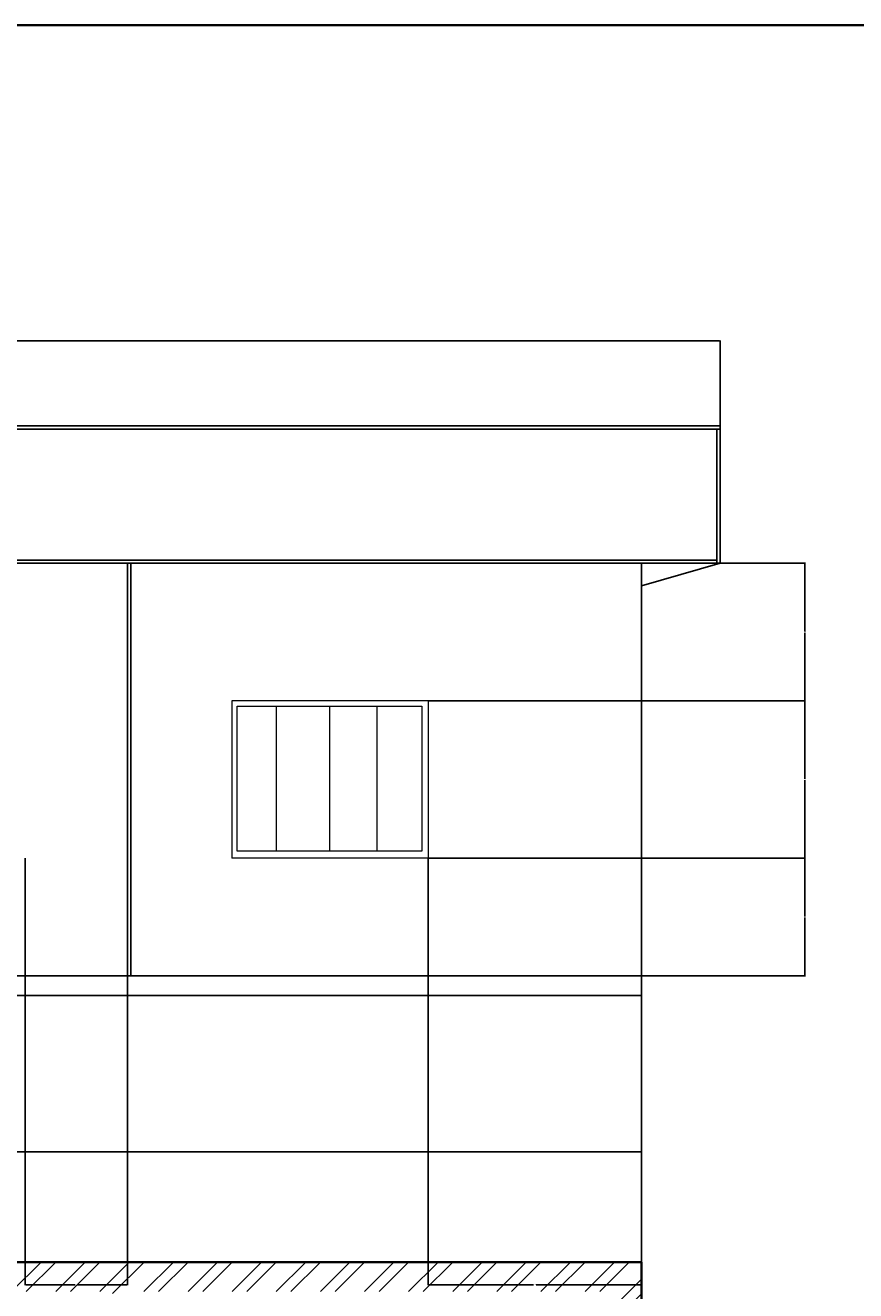
# Model space of a CAD drawing. Units: inches. Extents: x 1152 to 2588, y 1459 to 2618.
# Tile 14 of 17: x 1548 to 1802, y 2231 to 2618. Entities that reach past the tile are written whole.
import ezdxf

# ---------------------------------------------------------------- set-up
doc = ezdxf.new("R2010")
doc.units = ezdxf.units.IN
for name, color, linetype, lineweight in [('A-ANNO-DIMS', 2, 'Continuous', 18), ('A-ANNO-TTLB', 7, 'Continuous', 35), ('A-ELEV', 7, 'Continuous', 25), ('A-GLAZ', 4, 'Continuous', 18), ('A-WALL', 7, 'Continuous', 35), ('A-WALL-PATT', 8, 'Continuous', 13)]:
    doc.layers.add(name, color=color, linetype=linetype, lineweight=lineweight)
doc.styles.get("Standard").update_dxf_attribs({"font": 'arial.ttf'})
doc.dimstyles.get("Standard").update_dxf_attribs({"dimtxt": 0.18, "dimasz": 0.18, "dimexe": 0.18, "dimexo": 0.0625, "dimgap": 0.09, "dimtad": 0, "dimtih": 1, "dimtoh": 1, "dimdec": 4, "dimzin": 0, "dimdsep": 46, "dimtxsty": 'Standard', "dimcen": 0.09, "dimadec": 0, "dimazin": 0, "dimtfac": 1, "dimtdec": 4, "dimtofl": 0, "dimtmove": 0, "dimatfit": 3, "dimfxl": 1, "dimtolj": 1, "dimtzin": 0, "dimarcsym": 0})

# ---------------------------------------------------------------- blocks, each defined once
blk = doc.blocks.new('*D70')
at = {"layer": 'A-ANNO-DIMS', "color": 0, "lineweight": -2, "transparency": 16777216}
for p, q in [((1276.42, 2240.11), (1276.42, 2273.83)), ((1276.6, 2273.65), (1506.12, 2273.65)), ((1736.24, 2273.65), (1506.71, 2273.65)), ((1736.42, 2240.11), (1736.42, 2273.83))]:
    blk.add_line(p, q, dxfattribs=at)
at = {"layer": 'A-ANNO-DIMS', "color": 0, "transparency": 16777216}
for points in [[(1276.6, 2273.68), (1276.6, 2273.62), (1276.42, 2273.65)], [(1736.24, 2273.68), (1736.24, 2273.62), (1736.42, 2273.65)]]:
    blk.add_solid(points, dxfattribs=at)
at = {"layer": 'Defpoints', "color": 0, "transparency": 16777216}
for p in [(1736.42, 2273.65), (1276.42, 2240.05), (1736.42, 2240.05)]:
    blk.add_point(p, dxfattribs=at)
at = {"layer": 'A-ANNO-DIMS', "color": 0, "transparency": 16777216, "insert": (1506.42, 2273.65), "char_height": 0.18, "attachment_point": 5}
blk.add_mtext('\\A1;460', dxfattribs=at)
blk = doc.blocks.new('*D88')
at = {"layer": 'A-ANNO-DIMS', "color": 0, "lineweight": -2, "transparency": 16777216}
for p, q in [((1252.42, 2495.45), (1252.42, 2521.47)), ((1252.6, 2521.29), (1506.13, 2521.29)), ((1760.24, 2521.29), (1506.71, 2521.29)), ((1760.42, 2495.45), (1760.42, 2521.47))]:
    blk.add_line(p, q, dxfattribs=at)
at = {"layer": 'A-ANNO-DIMS', "color": 0, "transparency": 16777216}
for points in [[(1252.6, 2521.32), (1252.6, 2521.26), (1252.42, 2521.29)], [(1760.24, 2521.32), (1760.24, 2521.26), (1760.42, 2521.29)]]:
    blk.add_solid(points, dxfattribs=at)
at = {"layer": 'Defpoints', "color": 0, "transparency": 16777216}
for p in [(1760.42, 2521.29), (1252.42, 2495.39), (1760.42, 2495.39)]:
    blk.add_point(p, dxfattribs=at)
at = {"layer": 'A-ANNO-DIMS', "color": 0, "transparency": 16777216, "insert": (1506.42, 2521.29), "char_height": 0.18, "attachment_point": 5}
blk.add_mtext('\\A1;508', dxfattribs=at)
blk = doc.blocks.new('*D94')
at = {"layer": 'A-ANNO-DIMS', "color": 0, "lineweight": -2, "transparency": 16777216}
for p, q in [((1548.24, 2363.33), (1548.24, 2232.94)), ((1579.42, 2327.33), (1579.42, 2232.94)), ((1548.42, 2233.12), (1563.43, 2233.12)), ((1579.24, 2233.12), (1564.22, 2233.12))]:
    blk.add_line(p, q, dxfattribs=at)
at = {"layer": 'A-ANNO-DIMS', "color": 0, "transparency": 16777216}
for points in [[(1548.42, 2233.15), (1548.42, 2233.09), (1548.24, 2233.12)], [(1579.24, 2233.15), (1579.24, 2233.09), (1579.42, 2233.12)]]:
    blk.add_solid(points, dxfattribs=at)
at = {"layer": 'Defpoints', "color": 0, "transparency": 16777216}
for p in [(1548.24, 2363.39), (1579.42, 2327.39), (1579.42, 2233.12)]:
    blk.add_point(p, dxfattribs=at)
at = {"layer": 'A-ANNO-DIMS', "color": 0, "transparency": 16777216, "insert": (1563.83, 2233.12), "char_height": 0.18, "attachment_point": 5}
blk.add_mtext('\\A1;31.18', dxfattribs=at)
blk = doc.blocks.new('*D95')
at = {"layer": 'A-ANNO-DIMS', "color": 0, "lineweight": -2, "transparency": 16777216}
for p, q in [((1671.28, 2363.33), (1671.28, 2232.94)), ((1736.42, 2321.33), (1736.42, 2232.94)), ((1671.46, 2233.12), (1703.45, 2233.12)), ((1736.24, 2233.12), (1704.24, 2233.12))]:
    blk.add_line(p, q, dxfattribs=at)
at = {"layer": 'A-ANNO-DIMS', "color": 0, "transparency": 16777216}
for points in [[(1671.46, 2233.15), (1671.46, 2233.09), (1671.28, 2233.12)], [(1736.24, 2233.15), (1736.24, 2233.09), (1736.42, 2233.12)]]:
    blk.add_solid(points, dxfattribs=at)
at = {"layer": 'Defpoints', "color": 0, "transparency": 16777216}
for p in [(1671.28, 2363.39), (1736.42, 2321.39), (1736.42, 2233.12)]:
    blk.add_point(p, dxfattribs=at)
at = {"layer": 'A-ANNO-DIMS', "color": 0, "transparency": 16777216, "insert": (1703.85, 2233.12), "char_height": 0.18, "attachment_point": 5}
blk.add_mtext('\\A1;65.14', dxfattribs=at)
blk = doc.blocks.new('*D96')
at = {"layer": 'A-ANNO-DIMS', "color": 0, "lineweight": -2, "transparency": 16777216}
for p, q in [((1671.34, 2411.39), (1786.5, 2411.39)), ((1786.32, 2411.21), (1786.32, 2387.57)), ((1786.32, 2363.57), (1786.32, 2387.21)), ((1671.34, 2363.39), (1786.5, 2363.39))]:
    blk.add_line(p, q, dxfattribs=at)
at = {"layer": 'A-ANNO-DIMS', "color": 0, "transparency": 16777216}
for points in [[(1786.29, 2411.21), (1786.35, 2411.21), (1786.32, 2411.39)], [(1786.29, 2363.57), (1786.35, 2363.57), (1786.32, 2363.39)]]:
    blk.add_solid(points, dxfattribs=at)
at = {"layer": 'Defpoints', "color": 0, "transparency": 16777216}
for p in [(1671.28, 2411.39), (1786.32, 2411.39), (1671.28, 2363.39)]:
    blk.add_point(p, dxfattribs=at)
at = {"layer": 'A-ANNO-DIMS', "color": 0, "transparency": 16777216, "insert": (1786.32, 2387.39), "char_height": 0.18, "attachment_point": 5}
blk.add_mtext('\\A1;48', dxfattribs=at)
blk = doc.blocks.new('*D97')
at = {"layer": 'A-ANNO-DIMS', "color": 0, "lineweight": -2, "transparency": 16777216}
for p, q in [((1671.34, 2363.39), (1786.5, 2363.39)), ((1786.32, 2363.21), (1786.32, 2345.57)), ((1786.32, 2327.57), (1786.32, 2345.21)), ((1736.48, 2327.39), (1786.5, 2327.39))]:
    blk.add_line(p, q, dxfattribs=at)
at = {"layer": 'A-ANNO-DIMS', "color": 0, "transparency": 16777216}
for points in [[(1786.29, 2363.21), (1786.35, 2363.21), (1786.32, 2363.39)], [(1786.29, 2327.57), (1786.35, 2327.57), (1786.32, 2327.39)]]:
    blk.add_solid(points, dxfattribs=at)
at = {"layer": 'Defpoints', "color": 0, "transparency": 16777216}
for p in [(1671.28, 2363.39), (1786.32, 2363.39), (1736.42, 2327.39)]:
    blk.add_point(p, dxfattribs=at)
at = {"layer": 'A-ANNO-DIMS', "color": 0, "transparency": 16777216, "insert": (1786.32, 2345.39), "char_height": 0.18, "attachment_point": 5}
blk.add_mtext('\\A1;36', dxfattribs=at)
blk = doc.blocks.new('*D98')
at = {"layer": 'A-ANNO-DIMS', "color": 0, "lineweight": -2, "transparency": 16777216}
for p, q in [((1760.48, 2453.39), (1786.5, 2453.39)), ((1786.32, 2453.21), (1786.32, 2432.57)), ((1786.32, 2411.57), (1786.32, 2432.21)), ((1671.34, 2411.39), (1786.5, 2411.39))]:
    blk.add_line(p, q, dxfattribs=at)
at = {"layer": 'A-ANNO-DIMS', "color": 0, "transparency": 16777216}
for points in [[(1786.29, 2453.21), (1786.35, 2453.21), (1786.32, 2453.39)], [(1786.29, 2411.57), (1786.35, 2411.57), (1786.32, 2411.39)]]:
    blk.add_solid(points, dxfattribs=at)
at = {"layer": 'Defpoints', "color": 0, "transparency": 16777216}
for p in [(1760.42, 2453.39), (1786.32, 2453.39), (1671.28, 2411.39)]:
    blk.add_point(p, dxfattribs=at)
at = {"layer": 'A-ANNO-DIMS', "color": 0, "transparency": 16777216, "insert": (1786.32, 2432.39), "char_height": 0.18, "attachment_point": 5}
blk.add_mtext('\\A1;42', dxfattribs=at)

msp = doc.modelspace()

# ---------------------------------------------------------------- hatches: boundary and pattern name
at = {"layer": 'A-WALL-PATT'}
h = msp.add_hatch(dxfattribs=at)
h.set_pattern_fill('ANSI32', color=256)
h.paths.add_polyline_path([(1408.9272, 2240.0458), (1276.4165, 2240.0458), (1276.4165, 2192.7491), (1285.4165, 2192.7491), (1285.4165, 2231.0458), (1369.4165, 2231.0458), (1369.4165, 2084.0458), (1526.9165, 2084.0458), (1526.9165, 2096.3728), (1524.6665, 2096.3728), (1522.4165, 2096.3728), (1522.4165, 2093.0458), (1378.4165, 2093.0458), (1378.4165, 2231.0458), (1408.9272, 2231.0458)])
h.paths.add_polyline_path([(1736.4165, 2240.0458), (1468.9272, 2240.0458), (1468.9272, 2231.0458), (1522.4165, 2231.0458), (1522.4165, 2127.3313), (1526.9165, 2127.3313), (1526.9165, 2231.0458), (1574.9165, 2231.0458), (1574.9165, 2188.0458), (1579.4165, 2188.0458), (1579.4165, 2231.0458), (1727.4165, 2231.0458), (1727.4165, 2183.9728), (1736.4165, 2183.9728)])
h.paths.add_polyline_path([(1285.4165, 2156.7491), (1276.4165, 2156.7491), (1276.4165, 2084.0458), (1285.4165, 2084.0458)], flags=17)
h.paths.add_polyline_path([(1285.4165, 2043.5458), (1445.4165, 2043.5458), (1445.4165, 1943.6503), (1454.4165, 1943.6503), (1454.4165, 2048.0458), (1276.4165, 2048.0458), (1276.4165, 2019.2077), (1280.9165, 2019.2077), (1285.4165, 2019.2077)])
h.paths.add_polyline_path([(1285.4165, 1959.2077), (1276.4165, 1959.2077), (1276.4165, 1891.1319), (1280.9165, 1891.1319), (1285.4165, 1891.1319), (1285.4165, 1901.0458), (1376.8505, 1901.0458), (1376.8505, 1903.2958), (1376.8505, 1905.5458), (1285.4165, 1905.5458)])
h.paths.add_polyline_path([(1518.4165, 1905.5458), (1399.2832, 1905.5458), (1399.2832, 1903.2958), (1399.2832, 1901.0458), (1405.4165, 1901.0458), (1405.4165, 1884.8579), (1409.9165, 1884.8579), (1409.9165, 1901.0458), (1513.9165, 1901.0458), (1513.9165, 1869.1706), (1518.4165, 1869.1706)])
h.paths.add_polyline_path([(1520.5229, 1845.0458), (1518.4165, 1845.0458), (1518.4165, 1849.2927), (1516.1665, 1849.2927), (1513.9165, 1849.2927), (1513.9165, 1845.0458), (1409.9165, 1845.0458), (1409.9165, 1860.8579), (1405.4165, 1860.8579), (1405.4165, 1845.0458), (1285.4165, 1845.0458), (1285.4165, 1867.1319), (1276.4165, 1867.1319), (1276.4165, 1635.0458), (1285.4165, 1635.0458), (1285.4165, 1836.0458), (1405.4165, 1836.0458), (1405.4165, 1635.0458), (1414.4165, 1635.0458), (1424.7277, 1635.0458), (1424.7277, 1639.5458), (1424.7277, 1644.0458), (1414.4165, 1644.0458), (1414.4165, 1836.0458), (1414.4165, 1840.5831), (1520.5229, 1840.5831)])
h.paths.add_polyline_path([(1579.4165, 1840.5458), (1583.4035, 1840.5458), (1583.4035, 1845.0458), (1579.4165, 1845.0458), (1570.4165, 1845.0458), (1570.4165, 1840.5831), (1570.4165, 1644.0458), (1548.2359, 1644.0458), (1548.2359, 1635.0458), (1611.2801, 1635.0458), (1611.2801, 1639.5458), (1611.2801, 1644.0458), (1579.4165, 1644.0458)])
h.paths.add_polyline_path([(1488.2359, 1644.0458), (1472.0663, 1644.0458), (1472.0663, 1635.0458), (1488.2359, 1635.0458), (1488.2359, 1639.5458)], flags=17)
h.paths.add_polyline_path([(1736.4165, 1701.1863), (1727.4165, 1701.1863), (1727.4165, 1644.0458), (1671.2801, 1644.0458), (1671.2801, 1635.0458), (1736.4165, 1635.0458)])
h.paths.add_polyline_path([(1736.4165, 2147.9728), (1727.4165, 2147.9728), (1727.4165, 2093.0458), (1579.4165, 2093.0458), (1574.9165, 2093.0458), (1574.9165, 1971.6501), (1579.4165, 1971.6501), (1579.4165, 2084.0458), (1727.4165, 2084.0458), (1727.4165, 2054.3847), (1736.4165, 2054.3847)])
h.paths.add_polyline_path([(1736.4165, 1994.3847), (1727.4165, 1994.3847), (1727.4165, 1911.3562), (1736.4165, 1911.3562)])
h.paths.add_polyline_path([(1736.4165, 1875.3562), (1727.4165, 1875.3562), (1727.4165, 1845.0458), (1617.1767, 1845.0458), (1617.1767, 1842.7958), (1617.1767, 1840.5458), (1618.9165, 1840.5458), (1618.9165, 1788.5458), (1618.9165, 1784.0458), (1627.8699, 1784.0458), (1627.8699, 1788.5458), (1623.4165, 1788.5458), (1623.4165, 1840.5458), (1727.4165, 1840.5458), (1727.4165, 1828.7619), (1736.4165, 1828.7619)])
h.paths.add_polyline_path([(1727.4165, 1938.0458), (1579.4165, 1938.0458), (1579.4165, 1942.7722), (1574.9165, 1942.7722), (1574.9165, 1929.0458), (1727.4165, 1929.0458)])

# ---------------------------------------------------------------- linework, layer by layer
at = {"layer": 'A-ANNO-TTLB'}
msp.add_lwpolyline([(1152.3215, 2617.6685), (2587.6987, 2617.6685), (2587.6987, 1459.3148), (1152.3215, 1459.3148)], close=True, dxfattribs=at)
at = {"layer": 'A-ELEV'}
for p, q in [((1760.4165, 2495.3911), (1252.4165, 2495.3911)), ((1252.4165, 2494.3911), (1760.4165, 2494.3911)), ((1760.4165, 2494.3911), (1759.4165, 2494.3911)), ((1759.4165, 2494.3911), (1759.4165, 2453.3911)), ((1760.4165, 2453.3911), (1760.4165, 2495.3911)), ((1759.4165, 2454.3911), (1252.4165, 2454.3911)), ((1759.4165, 2453.3911), (1759.4165, 2454.3911)), ((1760.4165, 2453.3911), (1252.4165, 2453.3911)), ((1579.4165, 2453.3911), (1579.4165, 2327.3911)), ((1580.4165, 2327.3911), (1580.4165, 2453.3911)), ((1736.4165, 2453.3911), (1736.4165, 2321.3911)), ((1760.4165, 2453.3911), (1736.4165, 2446.4853)), ((1736.4165, 2327.3911), (1285.4165, 2327.3911)), ((1579.4165, 2327.3911), (1580.4165, 2327.3911)), ((1736.4165, 2321.3911), (1276.4165, 2321.3911))]:
    msp.add_line(p, q, dxfattribs=at)
at = {"layer": 'A-GLAZ'}
for p, q in [((1611.2801, 2411.3911), (1611.2801, 2363.3911)), ((1671.2801, 2411.3911), (1611.2801, 2411.3911)), ((1671.2801, 2411.3911), (1671.2801, 2363.3911)), ((1624.8254, 2409.8158), (1624.8254, 2365.4866)), ((1641.1403, 2409.8158), (1641.1403, 2365.4866)), ((1655.6366, 2409.8158), (1655.6366, 2365.4866)), ((1671.2801, 2363.3911), (1611.2801, 2363.3911))]:
    msp.add_line(p, q, dxfattribs=at)
msp.add_lwpolyline([(1612.96, 2409.8158), (1669.3206, 2409.8158), (1669.3206, 2365.4866), (1612.96, 2365.4866)], close=True, dxfattribs=at)
at = {"layer": 'A-WALL'}
for p, q in [((1276.4165, 2240.0458), (1736.4165, 2240.0458)), ((1736.4165, 2240.0458), (1736.4165, 1635.0458))]:
    msp.add_line(p, q, dxfattribs=at)

# ---------------------------------------------------------------- dimensions: what is measured, and where the dimension line sits
at = {"layer": 'A-ANNO-DIMS'}
for base, p1, p2, override, picture, middle in [((1760.4165, 2521.2911), (1252.4165, 2495.3911), (1760.4165, 2495.3911), {"dimdec": 0, "dimlfac": 1, "dimrnd": 0, "dimzin": 0, "dimdsep": 46, "dimlunit": 2}, '*D88', (1506.4165, 2521.2911)), ((1579.4165, 2233.12), (1548.2359, 2363.3911), (1579.4165, 2327.3911), {"dimdec": 2, "dimlfac": 1, "dimrnd": 0, "dimzin": 0, "dimdsep": 46, "dimlunit": 2}, '*D94', (1563.8262, 2233.12)), ((1736.4165, 2233.12), (1671.2801, 2363.3911), (1736.4165, 2321.3911), {"dimdec": 2, "dimlfac": 1, "dimrnd": 0, "dimzin": 0, "dimdsep": 46, "dimlunit": 2}, '*D95', (1703.8483, 2233.12)), ((1736.4165, 2273.6458), (1276.4165, 2240.0458), (1736.4165, 2240.0458), {"dimdec": 0, "dimlfac": 1, "dimrnd": 0, "dimzin": 0, "dimdsep": 46, "dimlunit": 2}, '*D70', (1506.4165, 2273.6458))]:
    dim = msp.add_linear_dim(base=base, p1=p1, p2=p2, dimstyle='Standard', override=override, dxfattribs=at)
    dim.commit()
    dim.dimension.update_dxf_attribs({"geometry": picture, "text_midpoint": middle})
for base, p1, p2, picture, middle in [((1786.3165, 2453.3911), (1671.2801, 2411.3911), (1760.4165, 2453.3911), '*D98', (1786.3165, 2432.3911)), ((1786.3165, 2411.3911), (1671.2801, 2363.3911), (1671.2801, 2411.3911), '*D96', (1786.3165, 2387.3911)), ((1786.3165, 2363.3911), (1736.4165, 2327.3911), (1671.2801, 2363.3911), '*D97', (1786.3165, 2345.3911))]:
    dim = msp.add_linear_dim(base=base, p1=p1, p2=p2, angle=90, dimstyle='Standard', override={"dimdec": 0, "dimlfac": 1, "dimrnd": 0, "dimzin": 0, "dimdsep": 46, "dimlunit": 2}, dxfattribs=at)
    dim.commit()
    dim.dimension.update_dxf_attribs({"geometry": picture, "text_midpoint": middle})

doc.saveas('drawing.dxf')
